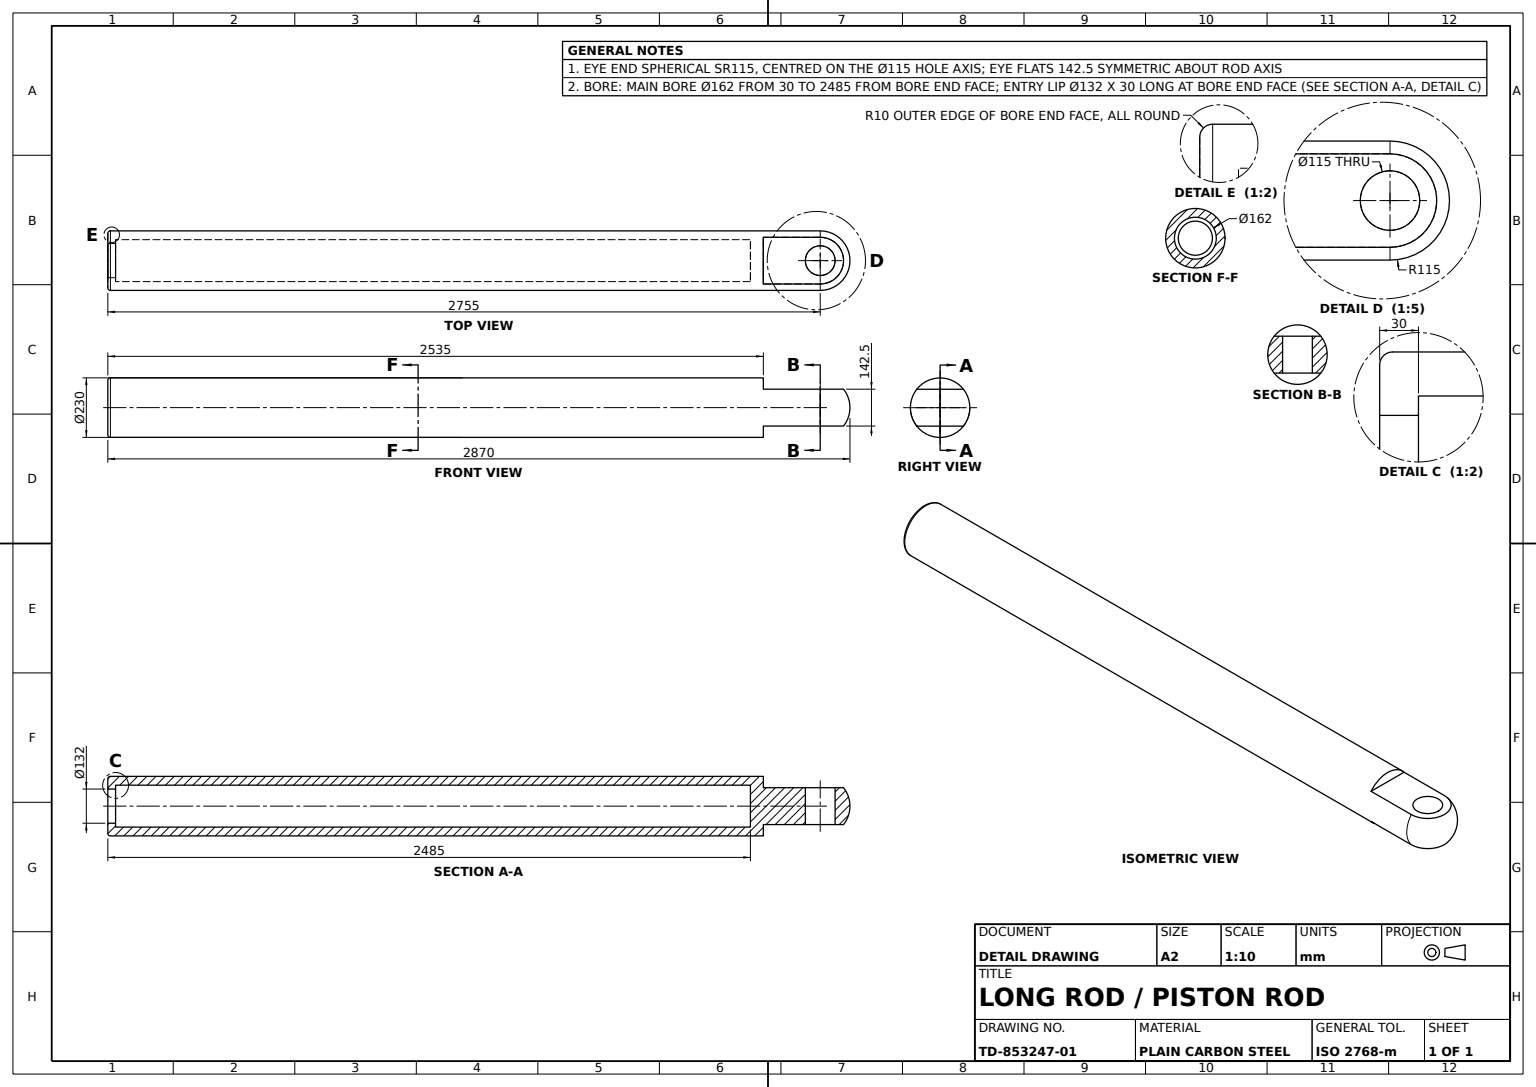
SolidWorks part; units mm, degrees
material "Plain Carbon Steel"
ref_plane "Front Plane" through (0, 0, 0) normal (0, 0, 1) x (1, 0, 0)
ref_plane "Top Plane" through (0, 0, 0) normal (0, 1, 0) x (1, 0, 0)
ref_plane "Right Plane" through (0, 0, 0) normal (1, 0, 0) x (0, 0, -1)
sketch "Barrel Profile Ø230 Sketch" plane through (0, 0, 0) normal (0, 0, 1) x (1, 0, 0)
  circle A0 centre (0, 0) radius 115
  dimension "D1" = 230
extrude "Barrel Body Ø230x2900" add sketch "Barrel Profile Ø230 Sketch" along normal mid plane 2900
sketch "End Trim Cut Sketch" plane through (0, 0, 0) normal (0, 1, 0) x (1, 0, 0)
  circle A0 centre (0, 1305) radius 57.5
  dimension "D1" = 115
  dimension "D2" = 1305
extrude "End Trim Cut" cut sketch "End Trim Cut Sketch" against normal mid plane 2900
sketch "Clevis Eye Profile Sketch" plane through (0, 0, 0) normal (1, 0, 0) x (0, 0, -1)
  line L0 (1450, 0) -> (417.7884, 0) construction
  line L1 (1450, -115) -> (1450, 115) construction
  line L2 (1085, -252.0838) -> (1085, -71.25)
  line L3 (1085, 252.0838) -> (1450, 252.0838)
  line L4 (1085, 252.0838) -> (1085, 71.25)
  line L5 (1085, 71.25) -> (1450, 71.25)
  line L6 (1450, 252.0838) -> (1450, 71.25)
  line L7 (1085, -71.25) -> (1450, -71.25)
  line L8 (1450, -252.0838) -> (1450, -71.25)
  line L9 (1085, -252.0838) -> (1450, -252.0838)
  dimension "D1" = 71.25
  dimension "D2" = 365
  dimension "D3" = 180.8338
extrude "Clevis Eye Profile Cut" cut sketch "Clevis Eye Profile Sketch" against normal mid plane 2900
sketch "Bore End Revolve Sketch" plane through (0, 0, 0) normal (0, 1, 0) x (1, 0, 0)
  line L0 (0, 1420) -> (0, 1537.1394) construction
  line L1 (0, 1537.1394) -> (209.0524, 1537.1394)
  line L2 (209.0524, 1537.1394) -> (209.0524, 1305)
  line L3 (209.0524, 1305) -> (115, 1305)
  line L4 (0, 1537.1394) -> (0, 1420)
  arc A0 (115, 1305) -> (0, 1420) centre (0, 1305) ccw
  dimension "D1" = 230
  dimension "D2" = 115
  dimension "D3" = 209.0524
  dimension "D4" = 232.1394
revolve "Bore End Revolved Cut" cut sketch "Bore End Revolve Sketch" angle 360 about L0
sketch "Eye End Revolve Sketch" plane through (0, 0, 0) normal (0, 1, 0) x (1, 0, 0)
  line L0 (0, -1450) -> (0, 1456.4541) construction
  line L1 (-115, -1450) -> (115, -1450) construction
  line L2 (0, -1450) -> (0, 1035)
  line L3 (66, -1450) -> (66, -1420)
  line L4 (66, -1420) -> (81, -1420)
  line L5 (81, -1420) -> (81, 1035)
  line L6 (90.2687, 1085) -> (-90.2687, 1085) construction
  line L7 (81, 1035) -> (0, 1035)
  line L8 (66, -1450) -> (0, -1450)
  dimension "D1" = 30
  dimension "D2" = 66
  dimension "D3" = 81
  dimension "D4" = 50
revolve "Eye End Revolved Cut" cut sketch "Eye End Revolve Sketch" angle 360 about L0
fillet "Edge Fillet R10" radius 10 1 edges at (115, 0, 1450)
